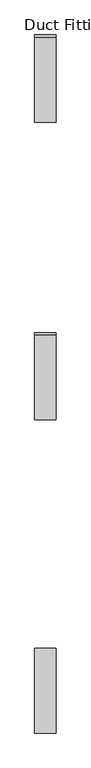
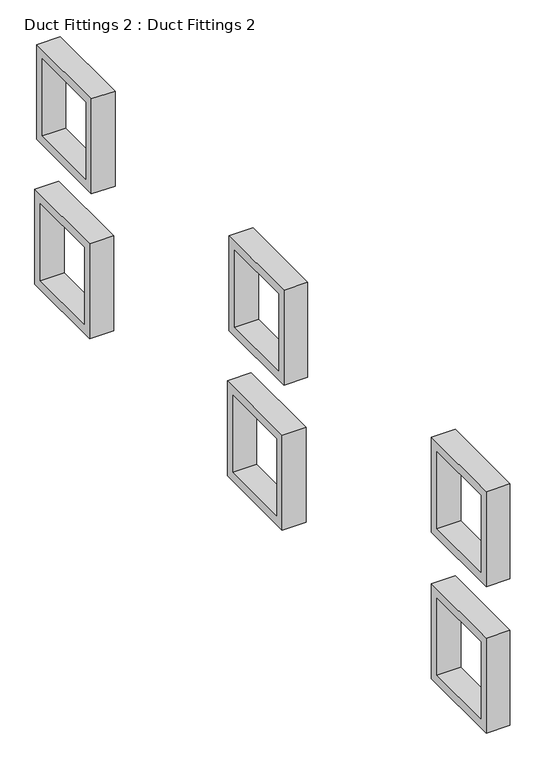
"""IFC4 building model written with IfcOpenShell, lengths in millimetres: duct fitting geometry, Duct Fittings 2 : Duct Fittings 2."""

from ifc_helpers import new_model, si_unit, frame, origin, place, context, project, spatial, polyline, outline, extrude, source, transform, mapped, element, save


def duct_fittings_2_duct_fittings_2_84becefd(model_context):
    return source(origin(), model_context, "Body", "SweptSolid", [
        extrude(outline(polyline([(-2974.6096146, 6654.8267455), (-2974.6096146, 5370.5543746), (-4188.4496146, 5370.5543746), (-4188.4496146, 6654.8267455), (-2974.6096146, 6654.8267455)]), holes=[polyline([(-3096.5296146, 6532.9067455), (-4066.5296146, 6532.9067455), (-4066.5296146, 5492.4743746), (-3096.5296146, 5492.4743746), (-3096.5296146, 6532.9067455)])]), frame((-2353.4667042, 0.0, 0.0), z_axis=(1.0, 0.0, 0.0), x_axis=(0.0, 1.0, 0.0)), (0.0, 0.0, 1.0), 304.8),
        extrude(outline(polyline([(1551.9653854, 6654.8267455), (1551.9653854, 5370.5543746), (338.1253854, 5370.5543746), (338.1253854, 6654.8267455), (1551.9653854, 6654.8267455)]), holes=[polyline([(1430.0453854, 6532.9067455), (460.0453854, 6532.9067455), (460.0453854, 5492.4743746), (1430.0453854, 5492.4743746), (1430.0453854, 6532.9067455)])]), frame((-2353.4667042, 0.0, 0.0), z_axis=(1.0, 0.0, 0.0), x_axis=(0.0, 1.0, 0.0)), (0.0, 0.0, 1.0), 304.8),
        extrude(outline(polyline([(5819.1653854, 6654.8267455), (5819.1653854, 5370.5543746), (4605.3253854, 5370.5543746), (4605.3253854, 6654.8267455), (5819.1653854, 6654.8267455)]), holes=[polyline([(5697.2453854, 6532.9067455), (4727.2453854, 6532.9067455), (4727.2453854, 5492.4743746), (5697.2453854, 5492.4743746), (5697.2453854, 6532.9067455)])]), frame((-2353.4667042, 0.0, 0.0), z_axis=(1.0, 0.0, 0.0), x_axis=(0.0, 1.0, 0.0)), (0.0, 0.0, 1.0), 304.8),
        extrude(outline(polyline([(5781.0653854, 8636.0267455), (5781.0653854, 7351.7543746), (4567.2253854, 7351.7543746), (4567.2253854, 8636.0267455), (5781.0653854, 8636.0267455)]), holes=[polyline([(5659.1453854, 8514.1067455), (4689.1453854, 8514.1067455), (4689.1453854, 7473.6743746), (5659.1453854, 7473.6743746), (5659.1453854, 8514.1067455)])]), frame((-2353.4667042, 0.0, 0.0), z_axis=(1.0, 0.0, 0.0), x_axis=(0.0, 1.0, 0.0)), (0.0, 0.0, 1.0), 304.8),
        extrude(outline(polyline([(1513.8653854, 8636.0267455), (1513.8653854, 7351.7543746), (300.0253854, 7351.7543746), (300.0253854, 8636.0267455), (1513.8653854, 8636.0267455)]), holes=[polyline([(1391.9453854, 8514.1067455), (421.9453854, 8514.1067455), (421.9453854, 7473.6743746), (1391.9453854, 7473.6743746), (1391.9453854, 8514.1067455)])]), frame((-2353.4667042, 0.0, 0.0), z_axis=(1.0, 0.0, 0.0), x_axis=(0.0, 1.0, 0.0)), (0.0, 0.0, 1.0), 304.8),
        extrude(outline(polyline([(-2974.6096146, 8636.0267455), (-2974.6096146, 7351.7543746), (-4188.4496146, 7351.7543746), (-4188.4496146, 8636.0267455), (-2974.6096146, 8636.0267455)]), holes=[polyline([(-3096.5296146, 8514.1067455), (-4066.5296146, 8514.1067455), (-4066.5296146, 7473.6743746), (-3096.5296146, 7473.6743746), (-3096.5296146, 8514.1067455)])]), frame((-2353.4667042, 0.0, 0.0), z_axis=(1.0, 0.0, 0.0), x_axis=(0.0, 1.0, 0.0)), (0.0, 0.0, 1.0), 304.8),
    ])


if __name__ == "__main__":
    model = new_model("IFC4")
    model_context = context("Model", 3, world=origin())
    ifc_project = project(units=[si_unit("LENGTHUNIT", "METRE", prefix="MILLI")], contexts=[model_context])
    site = spatial("IfcSite", under=ifc_project)
    building = spatial("IfcBuilding", under=site)
    placement = place(None, origin())
    duct_fittings_2_duct_fittings_2_shape = duct_fittings_2_duct_fittings_2_84becefd(model_context)
    element("IfcDuctFitting", 1, ObjectType="Duct Fittings 2 : Duct Fittings 2", at=placement, inside=building, context=model_context, shape_type="MappedRepresentation", body=[
        mapped(duct_fittings_2_duct_fittings_2_shape, transform((0.0, 0.0, 0.0), x_axis=(1.0, 0.0, 0.0), y_axis=(0.0, 1.0, 0.0), z_axis=(0.0, 0.0, 1.0))),
    ])
    save(model, "model.ifc")

# Revit data of these elements
# Element 1 (IfcDuctFitting, "Duct Fittings 2 : Duct Fittings 2")
#   Materials on its faces: "BB"
# Materials
#   "BB": class "Generic", colour RGB 24 76 198, transparency 0, Cost = 0
